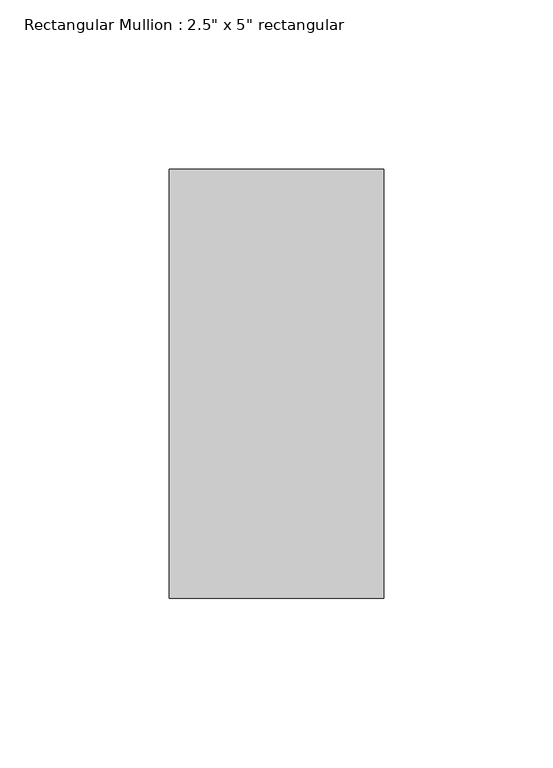
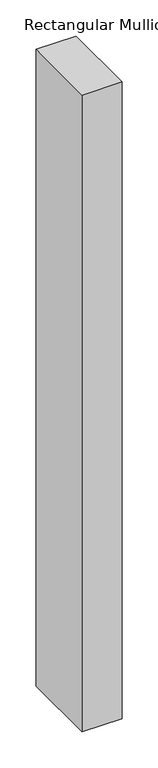
"""IFC4 building model written with IfcOpenShell, lengths in millimetres: member geometry."""

from ifc_helpers import new_model, si_unit, frame, origin, place, context, project, spatial, polyline, outline, extrude, source, transform, mapped, element, save


def member_be44f791(model_context):
    return source(origin(), model_context, "Body", "SweptSolid", [
        extrude(outline(polyline([(31.75, 63.5), (31.75, -63.5), (-31.75, -63.5), (-31.75, 63.5), (31.75, 63.5)])), frame((0.0, 0.0, -1073.1500002), z_axis=(0.0, 0.0, 1.0), x_axis=(1.0, 0.0, 0.0)), (0.0, 0.0, 1.0), 1073.1500002),
    ])


if __name__ == "__main__":
    model = new_model("IFC4")
    model_context = context("Model", 3, world=origin())
    ifc_project = project(units=[si_unit("LENGTHUNIT", "METRE", prefix="MILLI")], contexts=[model_context])
    site = spatial("IfcSite", under=ifc_project)
    building = spatial("IfcBuilding", under=site)
    placement = place(None, origin())
    member_shape = member_be44f791(model_context)
    element("IfcMember", 1, ObjectType="Rectangular Mullion : 2.5\" x 5\" rectangular", at=placement, inside=building, context=model_context, shape_type="MappedRepresentation", body=[
        mapped(member_shape, transform((0.0, 0.0, 0.0), x_axis=(1.0, 0.0, 0.0), y_axis=(0.0, 1.0, 0.0), z_axis=(0.0, 0.0, 1.0))),
    ])
    save(model, "model.ifc")

# Revit data of these elements
# Type "Rectangular Mullion : 2.5\" x 5\" rectangular"
#   built-in parameter 1007304 = 0.416667 (stored number, unit not read)
#   built-in parameter 1007301 = 0.104167 (stored number, unit not read)
#   built-in parameter 1007300 = 0.104167 (stored number, unit not read)
# Element 1 (IfcMember, "Rectangular Mullion : 2.5\" x 5\" rectangular")
#   Materials on its faces: "Aluminum"
# Materials
#   "Aluminum": class "Metal", colour RGB 247 247 247, transparency 0, Description = "Aluminum 6061", Cost = 0
